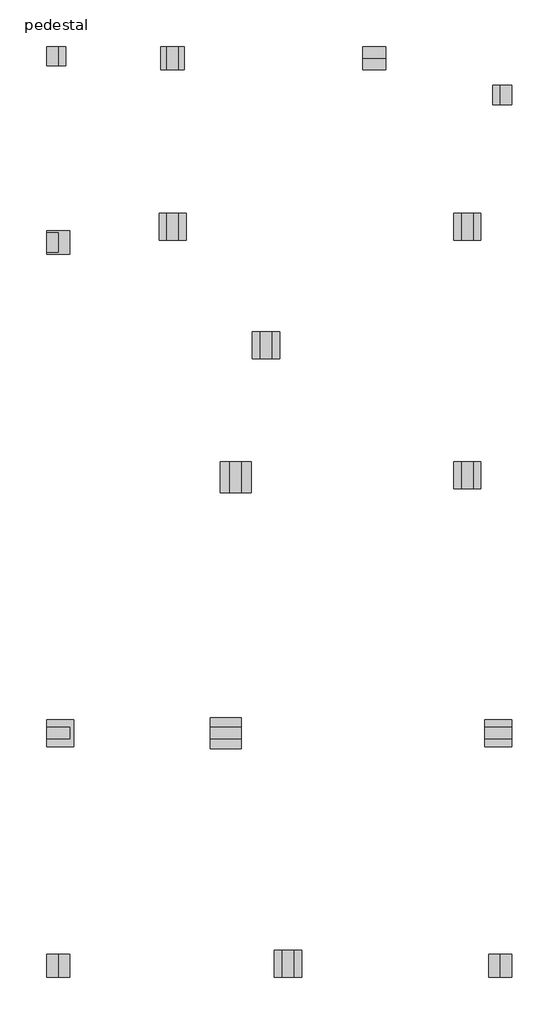
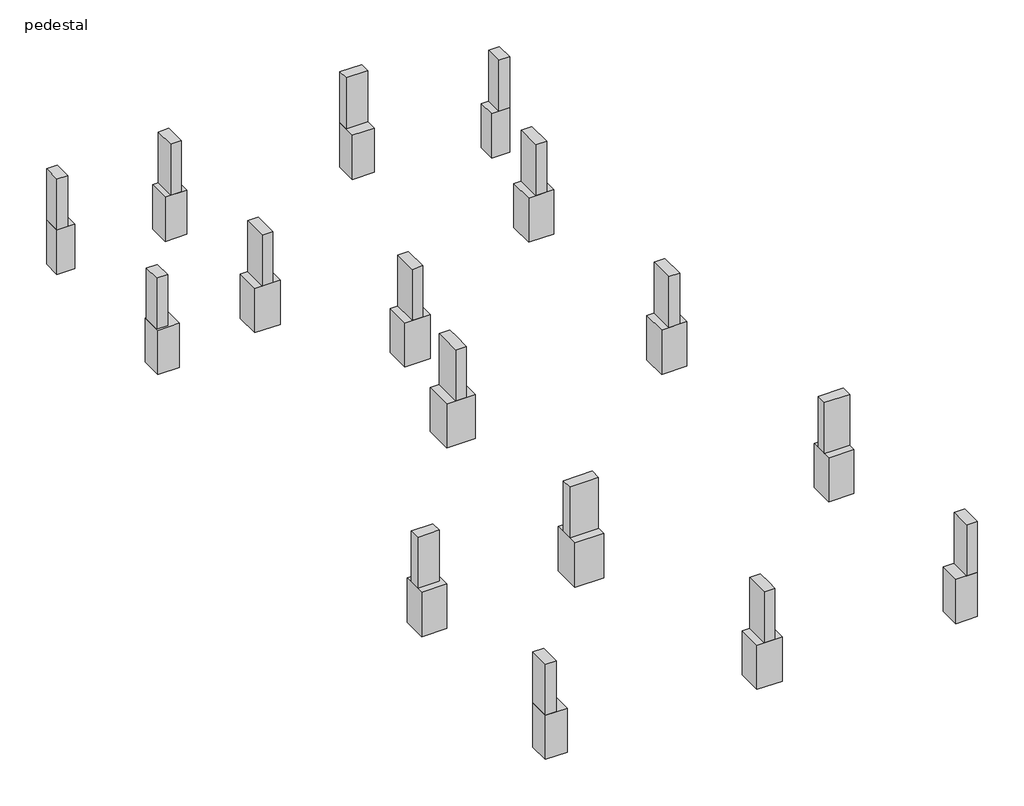
# One storey: 32 columns.
"""IFC4 building model written with IfcOpenShell, lengths in millimetres."""

from ifc_helpers import new_model, si_unit, frame, origin, place, context, project, spatial, polyline, outline, extrude, faceted_brep, transform, mapped, element, save
from components import column_96418790, column_547059a2, column_66439ef4, column_60b89d5c

model = new_model("IFC4")

# Units and contexts
model_context = context("Model", 3, world=origin())
ifc_project = project(units=[si_unit("LENGTHUNIT", "METRE", prefix="MILLI")], contexts=[model_context])

# Site, building, storey
site = spatial("IfcSite", under=ifc_project)
building = spatial("IfcBuilding", under=site)
storey = spatial("IfcBuildingStorey", under=building, Name="pedestal", Elevation=-1143.0)

# Columns
placement = place(None, origin())
element("IfcColumn", 1, ObjectType="M_Concrete-Rectangular-Column : 9\" x 15\"", at=placement, inside=storey, context=model_context, shape_type="SweptSolid", body=[
    extrude(outline(polyline([(17654.986814, 22575.1317951), (17883.586814, 22575.1317951), (17883.586814, 22194.1317951), (17654.986814, 22194.1317951), (17654.986814, 22575.1317951)])), frame((0.0, 0.0, -1143.0), z_axis=(0.0, 0.0, 1.0), x_axis=(1.0, 0.0, 0.0)), (0.0, 0.0, 1.0), 1143.0),
])
element("IfcColumn", 2, ObjectType="M_Concrete-Rectangular-Column : 9\" x 15\"", at=placement, inside=storey, context=model_context, shape_type="Brep", body=[
    faceted_brep([(17654.986814, 18917.5317951, -1143.0), (17883.586814, 18917.5317951, -1143.0), (17883.586814, 18536.5317951, -1143.0), (17654.986814, 18536.5317951, -1143.0), (17654.986814, 18917.5317951, 0.0), (17883.586814, 18917.5317951, 0.0), (17883.586814, 18917.5317951, -304.8), (17654.986814, 18917.5317951, -304.8), (17883.586814, 18536.5317951, 0.0), (17654.986814, 18536.5317951, 0.0)], [[[0, 1, 2, 3]], [[4, 5, 6, 1, 0, 7]], [[5, 8, 2, 1, 6]], [[8, 9, 3, 2]], [[9, 4, 7, 0, 3]], [[4, 9, 8, 5]]]),
])
element("IfcColumn", 3, ObjectType="M_Concrete-Rectangular-Column : 9\" x 15\"", at=placement, inside=storey, context=model_context, shape_type="Brep", body=[
    faceted_brep([(26570.386814, 21813.1317951, -1143.0), (26798.986814, 21813.1317951, -1143.0), (26798.986814, 21432.1317951, -1143.0), (26570.386814, 21432.1317951, -1143.0), (26570.386814, 21813.1317951, 0.0), (26798.986814, 21813.1317951, 0.0), (26570.386814, 21813.1317951, -304.8), (26798.986814, 21432.1317951, 0.0), (26570.386814, 21432.1317951, 0.0), (26570.386814, 21584.5317951, 0.0)], [[[0, 1, 2, 3]], [[4, 5, 1, 0, 6]], [[5, 7, 2, 1]], [[7, 8, 3, 2]], [[8, 9, 4, 6, 0, 3]], [[4, 9, 8, 7, 5]]]),
])
element("IfcColumn", 4, ObjectType="M_Concrete-Rectangular-Column : 9\" x 18\"", at=placement, inside=storey, context=model_context, shape_type="SweptSolid", body=[
    extrude(outline(polyline([(20245.786814, 22117.9317951), (20017.186814, 22117.9317951), (20017.186814, 22575.1317951), (20245.786814, 22575.1317951), (20245.786814, 22117.9317951)])), frame((0.0, 0.0, -1143.0), z_axis=(0.0, 0.0, 1.0), x_axis=(1.0, 0.0, 0.0)), (0.0, 0.0, 1.0), 1143.0),
])
element("IfcColumn", 5, ObjectType="M_Concrete-Rectangular-Column : 9\" x 18\"", at=placement, inside=storey, context=model_context, shape_type="SweptSolid", body=[
    extrude(outline(polyline([(24322.0020345, 22575.1317951), (24322.0020345, 22346.5317951), (23864.8020345, 22346.5317951), (23864.8020345, 22575.1317951), (24322.0020345, 22575.1317951)])), frame((0.0, 0.0, -1143.0), z_axis=(0.0, 0.0, 1.0), x_axis=(1.0, 0.0, 0.0)), (0.0, 0.0, 1.0), 1143.0),
])
element("IfcColumn", 6, ObjectType="M_Concrete-Rectangular-Column : 9\" x 18\"", at=placement, inside=storey, context=model_context, shape_type="SweptSolid", body=[
    extrude(outline(polyline([(18112.186814, 9202.0317951), (18112.186814, 8973.4317951), (17654.986814, 8973.4317951), (17654.986814, 9202.0317951), (18112.186814, 9202.0317951)])), frame((0.0, 0.0, -1143.0), z_axis=(0.0, 0.0, 1.0), x_axis=(1.0, 0.0, 0.0)), (0.0, 0.0, 1.0), 1143.0),
])
element("IfcColumn", 7, ObjectType="M_Concrete-Rectangular-Column : 9\" x 18\"", at=placement, inside=storey, context=model_context, shape_type="SweptSolid", body=[
    extrude(outline(polyline([(17654.986814, 4744.3317951), (17883.586814, 4744.3317951), (17883.586814, 4287.1317951), (17654.986814, 4287.1317951), (17654.986814, 4744.3317951)])), frame((0.0, 0.0, -1143.0), z_axis=(0.0, 0.0, 1.0), x_axis=(1.0, 0.0, 0.0)), (0.0, 0.0, 1.0), 1143.0),
])
element("IfcColumn", 8, ObjectType="M_Concrete-Rectangular-Column : 9\" x 18\"", at=placement, inside=storey, context=model_context, shape_type="SweptSolid", body=[
    extrude(outline(polyline([(26570.386814, 4744.3317951), (26798.986814, 4744.3317951), (26798.986814, 4287.1317951), (26570.386814, 4287.1317951), (26570.386814, 4744.3317951)])), frame((0.0, 0.0, -1143.0), z_axis=(0.0, 0.0, 1.0), x_axis=(1.0, 0.0, 0.0)), (0.0, 0.0, 1.0), 1143.0),
])
element("IfcColumn", 9, ObjectType="M_Concrete-Rectangular-Column : 9\" x 21\"", at=placement, inside=storey, context=model_context, shape_type="SweptSolid", body=[
    extrude(outline(polyline([(20017.186814, 19298.5317951), (20245.786814, 19298.5317951), (20245.786814, 18765.1317951), (20017.186814, 18765.1317951), (20017.186814, 19298.5317951)])), frame((0.0, 0.0, -1143.0), z_axis=(0.0, 0.0, 1.0), x_axis=(1.0, 0.0, 0.0)), (0.0, 0.0, 1.0), 1143.0),
])
element("IfcColumn", 10, ObjectType="M_Concrete-Rectangular-Column : 9\" x 21\"", at=placement, inside=storey, context=model_context, shape_type="SweptSolid", body=[
    extrude(outline(polyline([(25808.386814, 19298.5317951), (26036.986814, 19298.5317951), (26036.986814, 18765.1317951), (25808.386814, 18765.1317951), (25808.386814, 19298.5317951)])), frame((0.0, 0.0, -1143.0), z_axis=(0.0, 0.0, 1.0), x_axis=(1.0, 0.0, 0.0)), (0.0, 0.0, 1.0), 1143.0),
])
element("IfcColumn", 11, ObjectType="M_Concrete-Rectangular-Column : 9\" x 21\"", at=placement, inside=storey, context=model_context, shape_type="SweptSolid", body=[
    extrude(outline(polyline([(21851.7441916, 16974.4317951), (22080.3441916, 16974.4317951), (22080.3441916, 16441.0317951), (21851.7441916, 16441.0317951), (21851.7441916, 16974.4317951)])), frame((0.0, 0.0, -1143.0), z_axis=(0.0, 0.0, 1.0), x_axis=(1.0, 0.0, 0.0)), (0.0, 0.0, 1.0), 1143.0),
])
element("IfcColumn", 12, ObjectType="M_Concrete-Rectangular-Column : 9\" x 21\"", at=placement, inside=storey, context=model_context, shape_type="SweptSolid", body=[
    extrude(outline(polyline([(25808.386814, 14421.7317951), (26036.986814, 14421.7317951), (26036.986814, 13888.3317951), (25808.386814, 13888.3317951), (25808.386814, 14421.7317951)])), frame((0.0, 0.0, -1143.0), z_axis=(0.0, 0.0, 1.0), x_axis=(1.0, 0.0, 0.0)), (0.0, 0.0, 1.0), 1143.0),
])
element("IfcColumn", 13, ObjectType="M_Concrete-Rectangular-Column : 9\" x 21\"", at=placement, inside=storey, context=model_context, shape_type="Brep", body=[
    faceted_brep([(22284.136814, 4820.5317951, -1143.0), (22512.736814, 4820.5317951, -1143.0), (22512.736814, 4287.1317951, -1143.0), (22284.136814, 4287.1317951, -1143.0), (22284.136814, 4820.5317951, 0.0), (22512.736814, 4820.5317951, 0.0), (22512.736814, 4515.7317951, 0.0), (22512.736814, 4287.1317951, 0.0), (22512.736814, 4287.1317951, -304.8), (22284.136814, 4287.1317951, 0.0)], [[[0, 1, 2, 3]], [[4, 5, 1, 0]], [[5, 6, 7, 8, 2, 1]], [[7, 9, 3, 2, 8]], [[9, 4, 0, 3]], [[4, 9, 7, 6, 5]]]),
])
element("IfcColumn", 14, ObjectType="M_Concrete-Rectangular-Column : 9\" x 21\"", at=placement, inside=storey, context=model_context, shape_type="SweptSolid", body=[
    extrude(outline(polyline([(26265.586814, 8973.4317951), (26265.586814, 9202.0317951), (26798.986814, 9202.0317951), (26798.986814, 8973.4317951), (26265.586814, 8973.4317951)])), frame((0.0, 0.0, -1143.0), z_axis=(0.0, 0.0, 1.0), x_axis=(1.0, 0.0, 0.0)), (0.0, 0.0, 1.0), 1143.0),
])
element("IfcColumn", 15, ObjectType="M_Concrete-Rectangular-Column : 9\" x 24\"", at=placement, inside=storey, context=model_context, shape_type="SweptSolid", body=[
    extrude(outline(polyline([(20873.8441916, 9202.0317951), (21483.4441916, 9202.0317951), (21483.4441916, 8973.4317951), (20873.8441916, 8973.4317951), (20873.8441916, 9202.0317951)])), frame((0.0, 0.0, -1143.0), z_axis=(0.0, 0.0, 1.0), x_axis=(1.0, 0.0, 0.0)), (0.0, 0.0, 1.0), 1143.0),
])
element("IfcColumn", 16, ObjectType="M_Concrete-Rectangular-Column : 9\" x 24\"", at=placement, inside=storey, context=model_context, shape_type="Brep", body=[
    faceted_brep([(21254.8441916, 13812.1317951, -1143.0), (21254.8441916, 14421.7317951, -1143.0), (21483.4441916, 14421.7317951, -1143.0), (21483.4441916, 13812.1317951, -1143.0), (21254.8441916, 13812.1317951, 0.0), (21254.8441916, 14193.1317951, 0.0), (21254.8441916, 14421.7317951, 0.0), (21254.8441916, 14421.7317951, -304.8), (21483.4441916, 14421.7317951, 0.0), (21483.4441916, 14421.7317951, -304.8), (21483.4441916, 14193.1317951, 0.0), (21483.4441916, 13812.1317951, 0.0)], [[[0, 1, 2, 3]], [[4, 5, 6, 7, 1, 0]], [[6, 8, 9, 2, 1, 7]], [[8, 10, 11, 3, 2, 9]], [[11, 4, 0, 3]], [[4, 11, 10, 8, 6, 5]]]),
])
column_shape = column_96418790(model_context)
element("IfcColumn", 17, ObjectType="M_Concrete-Square-Column : 15\"", at=placement, inside=storey, context=model_context, shape_type="MappedRepresentation", body=[
    mapped(column_shape, transform((17845.486814, 22384.6317951, 0.0), x_axis=(1.0, 0.0, 0.0), y_axis=(0.0, 1.0, 0.0), z_axis=(0.0, 0.0, 1.0))),
])
element("IfcColumn", 18, ObjectType="M_Concrete-Square-Column : 15\"", at=placement, inside=storey, context=model_context, shape_type="MappedRepresentation", body=[
    mapped(column_shape, transform((26608.486814, 21622.6317951, 0.0), x_axis=(1.0, 0.0, 0.0), y_axis=(0.0, 1.0, 0.0), z_axis=(0.0, 0.0, 1.0))),
])
column_2_shape = column_547059a2(model_context)
element("IfcColumn", 19, ObjectType="M_Concrete-Square-Column : 18\"", at=placement, inside=storey, context=model_context, shape_type="MappedRepresentation", body=[
    mapped(column_2_shape, transform((20131.486814, 22346.5317951, 0.0), x_axis=(1.0, 0.0, 0.0), y_axis=(0.0, 1.0, 0.0), z_axis=(0.0, 0.0, 1.0))),
])
element("IfcColumn", 20, ObjectType="M_Concrete-Square-Column : 18\"", at=placement, inside=storey, context=model_context, shape_type="MappedRepresentation", body=[
    mapped(column_2_shape, transform((24093.4020345, 22346.5317951, 0.0), x_axis=(1.0, 0.0, 0.0), y_axis=(0.0, 1.0, 0.0), z_axis=(0.0, 0.0, 1.0))),
])
element("IfcColumn", 21, ObjectType="M_Concrete-Square-Column : 18\"", at=placement, inside=storey, context=model_context, shape_type="MappedRepresentation", body=[
    mapped(column_2_shape, transform((17883.586814, 18727.0317951, 0.0), x_axis=(1.0, 0.0, 0.0), y_axis=(0.0, 1.0, 0.0), z_axis=(0.0, 0.0, 1.0))),
])
element("IfcColumn", 22, ObjectType="M_Concrete-Square-Column : 18\"", at=placement, inside=storey, context=model_context, shape_type="MappedRepresentation", body=[
    mapped(column_2_shape, transform((17883.586814, 4515.7317951, 0.0), x_axis=(1.0, 0.0, 0.0), y_axis=(0.0, 1.0, 0.0), z_axis=(0.0, 0.0, 1.0))),
])
element("IfcColumn", 23, ObjectType="M_Concrete-Square-Column : 18\"", at=placement, inside=storey, context=model_context, shape_type="MappedRepresentation", body=[
    mapped(column_2_shape, transform((26570.386814, 4515.7317951, 0.0), x_axis=(1.0, 0.0, 0.0), y_axis=(0.0, 1.0, 0.0), z_axis=(0.0, 0.0, 1.0))),
])
column_3_shape = column_66439ef4(model_context)
element("IfcColumn", 24, ObjectType="M_Concrete-Square-Column : 21\"", at=placement, inside=storey, context=model_context, shape_type="MappedRepresentation", body=[
    mapped(column_3_shape, transform((20131.486814, 19031.8317951, 0.0), x_axis=(1.0, 0.0, 0.0), y_axis=(0.0, 1.0, 0.0), z_axis=(0.0, 0.0, 1.0))),
])
element("IfcColumn", 25, ObjectType="M_Concrete-Square-Column : 21\"", at=placement, inside=storey, context=model_context, shape_type="MappedRepresentation", body=[
    mapped(column_3_shape, transform((21966.0441916, 16707.7317951, 0.0), x_axis=(1.0, 0.0, 0.0), y_axis=(0.0, 1.0, 0.0), z_axis=(0.0, 0.0, 1.0))),
])
element("IfcColumn", 26, ObjectType="M_Concrete-Square-Column : 21\"", at=placement, inside=storey, context=model_context, shape_type="MappedRepresentation", body=[
    mapped(column_3_shape, transform((22398.436814, 4553.8317951, 0.0), x_axis=(1.0, 0.0, 0.0), y_axis=(0.0, 1.0, 0.0), z_axis=(0.0, 0.0, 1.0))),
])
column_4_shape = column_60b89d5c(model_context)
element("IfcColumn", 27, ObjectType="M_Concrete-Square-Column : 24\"", at=placement, inside=storey, context=model_context, shape_type="MappedRepresentation", body=[
    mapped(column_4_shape, transform((21369.1441916, 14116.9317951, 0.0), x_axis=(1.0, 0.0, 0.0), y_axis=(0.0, 1.0, 0.0), z_axis=(0.0, 0.0, 1.0))),
])
element("IfcColumn", 28, ObjectType="M_Concrete-Square-Column : 24\"", at=placement, inside=storey, context=model_context, shape_type="MappedRepresentation", body=[
    mapped(column_4_shape, transform((21178.6441916, 9087.7317951, 0.0), x_axis=(1.0, 0.0, 0.0), y_axis=(0.0, 1.0, 0.0), z_axis=(0.0, 0.0, 1.0))),
])
element("IfcColumn", 29, ObjectType="M_Concrete-Square-Column : f4 21\"", at=placement, inside=storey, context=model_context, shape_type="MappedRepresentation", body=[
    mapped(column_3_shape, transform((25922.686814, 19031.8317951, 0.0), x_axis=(1.0, 0.0, 0.0), y_axis=(0.0, 1.0, 0.0), z_axis=(0.0, 0.0, 1.0))),
])
element("IfcColumn", 30, ObjectType="M_Concrete-Square-Column : f4 21\"", at=placement, inside=storey, context=model_context, shape_type="MappedRepresentation", body=[
    mapped(column_3_shape, transform((25922.686814, 14155.0317951, 0.0), x_axis=(1.0, 0.0, 0.0), y_axis=(0.0, 1.0, 0.0), z_axis=(0.0, 0.0, 1.0))),
])
element("IfcColumn", 31, ObjectType="M_Concrete-Square-Column : sf2 21\"", at=placement, inside=storey, context=model_context, shape_type="MappedRepresentation", body=[
    mapped(column_3_shape, transform((17921.686814, 9087.7317951, 0.0), x_axis=(1.0, 0.0, 0.0), y_axis=(0.0, 1.0, 0.0), z_axis=(0.0, 0.0, 1.0))),
])
element("IfcColumn", 32, ObjectType="M_Concrete-Square-Column : sf2 21\"", at=placement, inside=storey, context=model_context, shape_type="MappedRepresentation", body=[
    mapped(column_3_shape, transform((26532.286814, 9087.7317951, 0.0), x_axis=(1.0, 0.0, 0.0), y_axis=(0.0, 1.0, 0.0), z_axis=(0.0, 0.0, 1.0))),
])

save(model, "model.ifc")

# Revit data of these elements
# Type "M_Concrete-Rectangular-Column : 9\" x 15\""
#   b = 381 mm
#   h = 228.6 mm
#   Structural Material [instance default] = Concrete, Cast-in-Place gray
# Type "M_Concrete-Rectangular-Column : 9\" x 18\""
#   b = 457.2 mm
#   h = 228.6 mm
#   Structural Material [instance default] = Concrete, Cast-in-Place gray
# Type "M_Concrete-Rectangular-Column : 9\" x 21\""
#   b = 533.4 mm
#   h = 228.6 mm
#   Structural Material [instance default] = Concrete, Cast-in-Place gray
# Type "M_Concrete-Rectangular-Column : 9\" x 24\""
#   b = 228.6 mm
#   h = 609.6 mm
#   Structural Material [instance default] = Concrete, Cast-in-Place gray
# Type "M_Concrete-Square-Column : 15\""
#   b = 381 mm
#   Structural Material [instance default] = Concrete, Cast-in-Place gray
# Type "M_Concrete-Square-Column : 18\""
#   b = 457.2 mm
#   Structural Material [instance default] = Concrete, Cast-in-Place gray
# Type "M_Concrete-Square-Column : 21\""
#   b = 533.4 mm
#   Structural Material [instance default] = Concrete, Cast-in-Place gray
# Type "M_Concrete-Square-Column : 24\""
#   b = 609.6 mm
#   Structural Material [instance default] = Concrete, Cast-in-Place gray
# Type "M_Concrete-Square-Column : f4 21\""
#   b = 533.4 mm
#   Structural Material [instance default] = Concrete, Cast-in-Place gray
# Type "M_Concrete-Square-Column : sf2 21\""
#   b = 533.4 mm
#   Structural Material [instance default] = Concrete, Cast-in-Place gray
# Elements 1, 2, 3 (IfcColumn, "M_Concrete-Rectangular-Column : 9\" x 15\"")
#   Structural Material = Concrete, Cast-in-Place gray
#   Phase Created = New Construction
#   Materials on its faces: "Concrete, Cast-in-Place gray"
# Elements 4, 5, 6, 7, 8 (IfcColumn, "M_Concrete-Rectangular-Column : 9\" x 18\"")
#   Structural Material = Concrete, Cast-in-Place gray
#   Phase Created = New Construction
#   Materials on its faces: "Concrete, Cast-in-Place gray"
# Elements 9, 10, 11, 12, 13, 14 (IfcColumn, "M_Concrete-Rectangular-Column : 9\" x 21\"")
#   Structural Material = Concrete, Cast-in-Place gray
#   Phase Created = New Construction
#   Materials on its faces: "Concrete, Cast-in-Place gray"
# Elements 15, 16 (IfcColumn, "M_Concrete-Rectangular-Column : 9\" x 24\"")
#   Structural Material = Concrete, Cast-in-Place gray
#   Phase Created = New Construction
#   Materials on its faces: "Concrete, Cast-in-Place gray"
# Elements 17, 18 (IfcColumn, "M_Concrete-Square-Column : 15\"")
#   Structural Material = Concrete, Cast-in-Place gray
#   Phase Created = New Construction
#   Materials on its faces: "Concrete, Cast-in-Place gray"
# Elements 19, 20, 21, 22, 23 (IfcColumn, "M_Concrete-Square-Column : 18\"")
#   Structural Material = Concrete, Cast-in-Place gray
#   Phase Created = New Construction
#   Materials on its faces: "Concrete, Cast-in-Place gray"
# Elements 24, 25, 26 (IfcColumn, "M_Concrete-Square-Column : 21\"")
#   Structural Material = Concrete, Cast-in-Place gray
#   Phase Created = New Construction
#   Materials on its faces: "Concrete, Cast-in-Place gray"
# Elements 27, 28 (IfcColumn, "M_Concrete-Square-Column : 24\"")
#   Structural Material = Concrete, Cast-in-Place gray
#   Phase Created = New Construction
#   Materials on its faces: "Concrete, Cast-in-Place gray"
# Elements 29, 30 (IfcColumn, "M_Concrete-Square-Column : f4 21\"")
#   Structural Material = Concrete, Cast-in-Place gray
#   Phase Created = New Construction
#   Materials on its faces: "Concrete, Cast-in-Place gray"
# Elements 31, 32 (IfcColumn, "M_Concrete-Square-Column : sf2 21\"")
#   Structural Material = Concrete, Cast-in-Place gray
#   Phase Created = New Construction
#   Materials on its faces: "Concrete, Cast-in-Place gray"
# Materials
#   "Concrete, Cast-in-Place gray": class "Concrete", colour RGB 192 192 192, transparency 0, Description = "Cast-in-place concrete", Cost = 0
